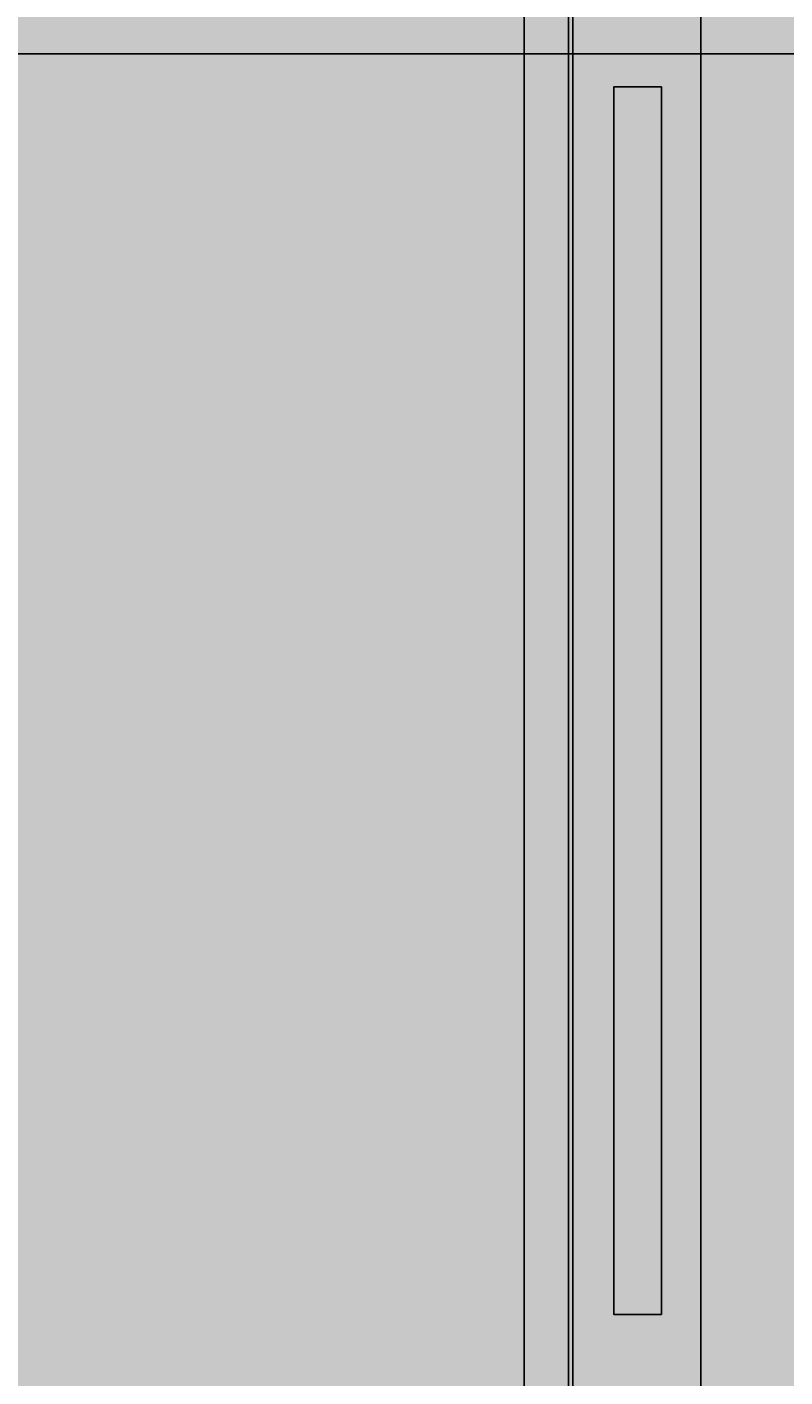
# Model space of a CAD drawing. Units: feet. Extents: x 2695 to 2912, y 795 to 1139.
# Tile 22 of 83: x 2791 to 2808, y 845 to 875. Entities that reach past the tile are written whole.
import ezdxf

# ---------------------------------------------------------------- set-up
doc = ezdxf.new("R2010")
doc.units = ezdxf.units.FT
for name, color, linetype, lineweight in [('A-ANNO-DIMS', 2, 'Continuous', 18), ('A-DOOR', 3, 'Continuous', 25), ('A-DOOR-PATT', 33, 'Continuous', 13), ('A-ELEV-PATT', 252, 'Continuous', 13)]:
    doc.layers.add(name, color=color, linetype=linetype, lineweight=lineweight)
doc.styles.get("Standard").update_dxf_attribs({"font": 'arial.ttf'})
doc.dimstyles.get("Standard").update_dxf_attribs({"dimtxt": 0.18, "dimasz": 0.18, "dimexe": 0.18, "dimexo": 0.0625, "dimgap": 0.09, "dimtad": 0, "dimtih": 1, "dimtoh": 1, "dimdec": 1, "dimzin": 0, "dimdsep": 46, "dimlunit": 3, "dimtxsty": 'Standard', "dimcen": 0.09, "dimadec": 0, "dimazin": 0, "dimtfac": 1, "dimtdec": 1, "dimtofl": 0, "dimtmove": 0, "dimatfit": 3, "dimfxl": 1, "dimtolj": 1, "dimtzin": 0, "dimarcsym": 0})

# ---------------------------------------------------------------- blocks, each defined once
blk = doc.blocks.new('*D13')
at = {"layer": 'A-ANNO-DIMS', "color": 0, "lineweight": -2, "transparency": 16777216}
for p, q in [((2758.214, 874.857), (2911.424, 874.857)), ((2911.244, 874.677), (2911.244, 843.076)), ((2911.244, 811.111), (2911.244, 842.712)), ((2890.699, 810.931), (2911.424, 810.931))]:
    blk.add_line(p, q, dxfattribs=at)
at = {"layer": 'A-ANNO-DIMS', "color": 0, "transparency": 16777216}
for points in [[(2911.214, 874.677), (2911.274, 874.677), (2911.244, 874.857)], [(2911.214, 811.111), (2911.274, 811.111), (2911.244, 810.931)]]:
    blk.add_solid(points, dxfattribs=at)
at = {"layer": 'Defpoints', "color": 0, "transparency": 16777216}
for p in [(2758.151, 874.857), (2911.244, 874.857), (2890.636, 810.931)]:
    blk.add_point(p, dxfattribs=at)
at = {"layer": 'A-ANNO-DIMS', "color": 0, "transparency": 16777216, "insert": (2911.244, 842.894), "char_height": 0.18, "attachment_point": 5}
blk.add_mtext('\\A1;63.93', dxfattribs=at)
blk = doc.blocks.new('*D14')
at = {"layer": 'A-ANNO-DIMS', "color": 0, "lineweight": -2, "transparency": 16777216}
for p, q in [((2838.439, 905.514), (2911.424, 905.514)), ((2911.244, 905.334), (2911.244, 890.368)), ((2911.244, 875.037), (2911.244, 890.004)), ((2758.214, 874.857), (2911.424, 874.857))]:
    blk.add_line(p, q, dxfattribs=at)
at = {"layer": 'A-ANNO-DIMS', "color": 0, "transparency": 16777216}
for points in [[(2911.214, 905.334), (2911.274, 905.334), (2911.244, 905.514)], [(2911.214, 875.037), (2911.274, 875.037), (2911.244, 874.857)]]:
    blk.add_solid(points, dxfattribs=at)
at = {"layer": 'Defpoints', "color": 0, "transparency": 16777216}
for p in [(2838.377, 905.514), (2911.244, 905.514), (2758.151, 874.857)]:
    blk.add_point(p, dxfattribs=at)
at = {"layer": 'A-ANNO-DIMS', "color": 0, "transparency": 16777216, "insert": (2911.244, 890.186), "char_height": 0.18, "attachment_point": 5}
blk.add_mtext('\\A1;30.66', dxfattribs=at)

msp = doc.modelspace()

# ---------------------------------------------------------------- hatches: boundary and pattern name
at = {"layer": 'A-DOOR-PATT'}
h = msp.add_hatch(color=256, dxfattribs=at)
h.set_gradient(color1=(211, 185, 150), color2=(211, 185, 150))
h.paths.add_polyline_path([(2805.9398, 905.5143), (2773.5029, 905.5143), (2773.5029, 810.9306), (2776.4999, 810.9306), (2776.4999, 902.5174), (2802.9429, 902.5174), (2802.9429, 810.9306), (2805.9398, 810.9306)])
h.paths.add_polyline_path([(2803.9681, 874.1057), (2805.0538, 874.1057), (2805.0538, 846.2857), (2803.9681, 846.2857)], flags=16)
h.paths.add_polyline_path([(2838.3767, 905.5143), (2805.9398, 905.5143), (2805.9398, 810.9306), (2808.9368, 810.9306), (2808.9368, 902.5174), (2835.3798, 902.5174), (2835.3798, 810.9306), (2838.3767, 810.9306)])
h = msp.add_hatch(color=256, dxfattribs=at)
h.set_gradient(color1=(211, 185, 150), color2=(211, 185, 150))
h.paths.add_polyline_path([(2777.5029, 901.5143), (2801.9398, 901.5143), (2801.9398, 810.9306), (2802.9429, 810.9306), (2802.9429, 902.5174), (2776.4999, 902.5174), (2776.4999, 810.9306), (2777.5029, 810.9306)])
h.paths.add_polyline_path([(2809.9398, 901.5143), (2834.3767, 901.5143), (2834.3767, 810.9306), (2835.3798, 810.9306), (2835.3798, 902.5174), (2808.9368, 902.5174), (2808.9368, 810.9306), (2809.9398, 810.9306)])
h = msp.add_hatch(color=256, dxfattribs=at)
h.set_gradient(color1=(173, 221, 247), color2=(173, 221, 247))
h.paths.add_polyline_path([(2801.9398, 901.5143), (2777.5029, 901.5143), (2777.5029, 810.9306), (2801.9398, 810.9306)])
h.paths.add_polyline_path([(2834.3767, 901.5143), (2809.9398, 901.5143), (2809.9398, 810.9306), (2834.3767, 810.9306)])
at = {"layer": 'A-ELEV-PATT'}
h = msp.add_hatch(color=256, dxfattribs=at)
h.set_gradient(color2=(0, 0, 0), tint=1)
h.paths.add_polyline_path([(2772.5216, 971.9673), (2770.6361, 971.9673), (2770.6361, 970.7156), (2772.5216, 970.7156)])
h.paths.add_polyline_path([(2773.2702, 971.9673), (2772.5216, 971.9673), (2772.5216, 970.7156), (2773.2702, 970.7156)])
h.paths.add_polyline_path([(2778.0341, 971.9673), (2773.2702, 971.9673), (2773.2702, 970.7156), (2778.0341, 970.7156)])
h.paths.add_polyline_path([(2780.0341, 971.9673), (2778.0341, 971.9673), (2778.0341, 970.7156), (2780.0341, 970.7156)])
h.paths.add_polyline_path([(2841.575, 971.9673), (2780.0341, 971.9673), (2780.0341, 970.7156), (2841.575, 970.7156)])
h.paths.add_polyline_path([(2843.575, 971.9673), (2841.575, 971.9673), (2841.575, 970.7156), (2843.575, 970.7156)])
h.paths.add_polyline_path([(2888.1882, 971.9673), (2843.575, 971.9673), (2843.575, 970.7156), (2888.1882, 970.7156)])
h.paths.add_polyline_path([(2888.9368, 971.9673), (2888.1882, 971.9673), (2888.1882, 970.7156), (2888.9368, 970.7156)], flags=17)
h.paths.add_polyline_path([(2890.6361, 971.9673), (2888.9368, 971.9673), (2888.9368, 970.7156), (2890.6361, 970.7156)])
h.paths.add_polyline_path([(2888.9368, 971.9673), (2888.1882, 971.9673), (2888.1882, 964.8267), (2888.9368, 964.8267)])
h.paths.add_polyline_path([(2888.9368, 964.8267), (2888.1882, 964.8267), (2888.1882, 964.1328), (2888.9368, 964.1328)])
h.paths.add_polyline_path([(2890.6361, 964.8267), (2888.9368, 964.8267), (2888.9368, 964.1328), (2890.6361, 964.1328)])
h.paths.add_polyline_path([(2888.1882, 964.8267), (2770.6361, 964.8267), (2770.6361, 964.1328), (2888.1882, 964.1328)])
h.paths.add_polyline_path([(2888.9368, 964.1328), (2888.1882, 964.1328), (2888.1882, 936.9306), (2888.9368, 936.9306)])
h.paths.add_polyline_path([(2890.6361, 956.614), (2888.9368, 956.614), (2888.9368, 955.9202), (2890.6361, 955.9202)])
h.paths.add_polyline_path([(2888.1882, 956.614), (2770.6361, 956.614), (2770.6361, 955.9202), (2888.1882, 955.9202)])
h.paths.add_polyline_path([(2890.6361, 949.2892), (2888.9368, 949.2892), (2888.9368, 948.5954), (2890.6361, 948.5954)])
h.paths.add_polyline_path([(2888.1882, 949.2892), (2770.6361, 949.2892), (2770.6361, 948.5954), (2888.1882, 948.5954)])
h.paths.add_polyline_path([(2890.6361, 941.3507), (2888.9368, 941.3507), (2888.9368, 940.6569), (2890.6361, 940.6569)])
h.paths.add_polyline_path([(2888.1882, 941.3507), (2770.6361, 941.3507), (2770.6361, 940.6569), (2888.1882, 940.6569)])
h.paths.add_polyline_path([(2773.2702, 970.7156), (2772.5216, 970.7156), (2772.5216, 964.8267), (2773.2702, 964.8267)])
h.paths.add_polyline_path([(2773.2702, 964.1328), (2772.5216, 964.1328), (2772.5216, 956.614), (2773.2702, 956.614)])
h.paths.add_polyline_path([(2773.2702, 955.9202), (2772.5216, 955.9202), (2772.5216, 936.9306), (2773.2702, 936.9306)])
h.paths.add_polyline_path([(2810.7893, 970.7156), (2810.0407, 970.7156), (2810.0407, 964.8267), (2810.7893, 964.8267)], flags=17)
h.paths.add_polyline_path([(2810.7893, 964.1328), (2810.0407, 964.1328), (2810.0407, 956.614), (2810.7893, 956.614)], flags=17)
h.paths.add_polyline_path([(2810.7893, 955.9202), (2810.0407, 955.9202), (2810.0407, 949.2892), (2810.7893, 949.2892)], flags=17)
h.paths.add_polyline_path([(2810.7893, 971.9673), (2810.0407, 971.9673), (2810.0407, 941.3507), (2810.7893, 941.3507)])
h.paths.add_polyline_path([(2810.7893, 940.6569), (2810.0407, 940.6569), (2810.0407, 936.9306), (2810.7893, 936.9306)])
h.paths.add_polyline_path([(2780.0341, 1018.8235), (2841.575, 1018.8235), (2841.575, 971.9673), (2843.575, 971.9673), (2843.575, 1020.8235), (2778.0341, 1020.8235), (2778.0341, 971.9673), (2780.0341, 971.9673)])
h.paths.add_polyline_path([(2780.0341, 970.7156), (2778.0341, 970.7156), (2778.0341, 964.8267), (2780.0341, 964.8267)])
h.paths.add_polyline_path([(2780.0341, 964.1328), (2778.0341, 964.1328), (2778.0341, 956.614), (2780.0341, 956.614)])
h.paths.add_polyline_path([(2780.0341, 955.9202), (2778.0341, 955.9202), (2778.0341, 949.2892), (2780.0341, 949.2892)])
h.paths.add_polyline_path([(2780.0341, 948.5954), (2778.0341, 948.5954), (2778.0341, 941.3507), (2780.0341, 941.3507)])
h.paths.add_polyline_path([(2780.0341, 940.6569), (2778.0341, 940.6569), (2778.0341, 936.9306), (2780.0341, 936.9306)])
h.paths.add_polyline_path([(2843.575, 940.6569), (2841.575, 940.6569), (2841.575, 936.9306), (2843.575, 936.9306)])
h.paths.add_polyline_path([(2843.575, 948.5954), (2841.575, 948.5954), (2841.575, 941.3507), (2843.575, 941.3507)])
h.paths.add_polyline_path([(2843.575, 970.7156), (2841.575, 970.7156), (2841.575, 964.8267), (2843.575, 964.8267)])
h.paths.add_polyline_path([(2843.575, 964.1328), (2841.575, 964.1328), (2841.575, 956.614), (2843.575, 956.614)])
h.paths.add_polyline_path([(2843.575, 955.9202), (2841.575, 955.9202), (2841.575, 949.2892), (2843.575, 949.2892)])
h.paths.add_polyline_path([(2805.0538, 874.1057), (2803.9681, 874.1057), (2803.9681, 846.2857), (2805.0538, 846.2857)])
h.paths.add_polyline_path([(2758.1515, 902.577), (2724.1893, 902.577), (2724.1893, 874.8571), (2758.1515, 874.8571)])
h.paths.add_polyline_path([(2726.1893, 900.577), (2756.1515, 900.577), (2756.1515, 876.8571), (2726.1893, 876.8571)], flags=16)
h.paths.add_polyline_path([(2740.7302, 900.577), (2741.6105, 900.577), (2741.6105, 876.8571), (2740.7302, 876.8571)], flags=0)

# ---------------------------------------------------------------- linework, layer by layer
at = {"layer": 'A-DOOR'}
for points in [[(2773.5029, 810.9306), (2773.5029, 905.5143), (2805.9398, 905.5143), (2805.9398, 810.9306)], [(2838.3767, 810.9306), (2838.3767, 905.5143), (2805.9398, 905.5143), (2805.9398, 810.9306)], [(2776.4999, 810.9306), (2776.4999, 902.5174), (2802.9429, 902.5174), (2802.9429, 810.9306)], [(2777.5029, 810.9306), (2777.5029, 901.5143), (2801.9398, 901.5143), (2801.9398, 810.9306)]]:
    msp.add_lwpolyline(points, dxfattribs=at)
for points in [[(2805.9398, 905.5143), (2805.9398, 905.5143), (2805.9398, 810.9306), (2805.9398, 810.9306)], [(2776.4999, 902.5174), (2803.0393, 902.5174), (2803.0393, 810.9306), (2776.4999, 810.9306)], [(2777.5029, 901.5143), (2801.9398, 901.5143), (2801.9398, 810.9306), (2777.5029, 810.9306)], [(2805.0538, 846.2857), (2803.9681, 846.2857), (2803.9681, 874.1057), (2805.0538, 874.1057)]]:
    msp.add_lwpolyline(points, close=True, dxfattribs=at)

# ---------------------------------------------------------------- dimensions: what is measured, and where the dimension line sits
at = {"layer": 'A-ANNO-DIMS'}
for base, p1, p2, picture, middle in [((2911.2444, 905.5143), (2758.1515, 874.8571), (2838.3767, 905.5143), '*D14', (2911.2444, 890.1857)), ((2911.2444, 874.8571), (2890.6361, 810.9306), (2758.1515, 874.8571), '*D13', (2911.2444, 842.8938))]:
    dim = msp.add_linear_dim(base=base, p1=p1, p2=p2, angle=90, dimstyle='Standard', override={"dimdec": 2, "dimlfac": 1, "dimrnd": 0, "dimzin": 0, "dimdsep": 46, "dimlunit": 2}, dxfattribs=at)
    dim.commit()
    dim.dimension.update_dxf_attribs({"geometry": picture, "text_midpoint": middle})

doc.saveas('drawing.dxf')
